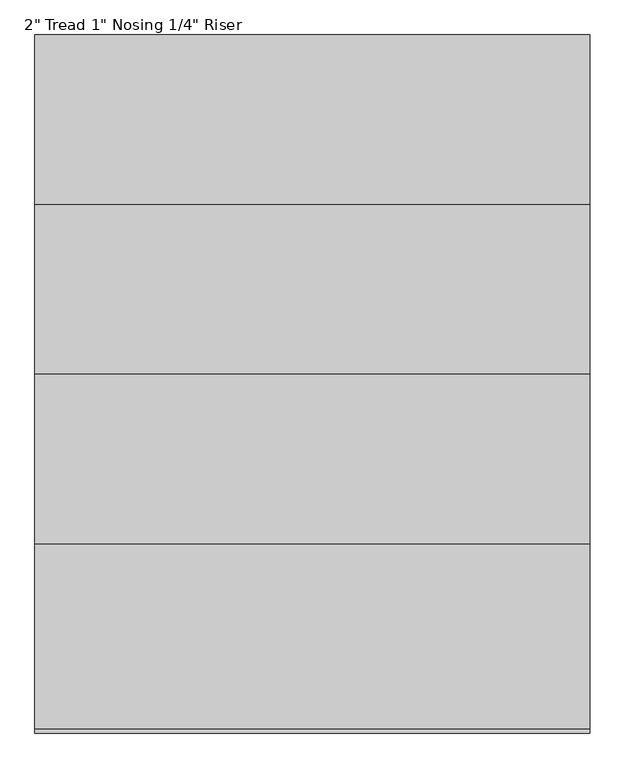
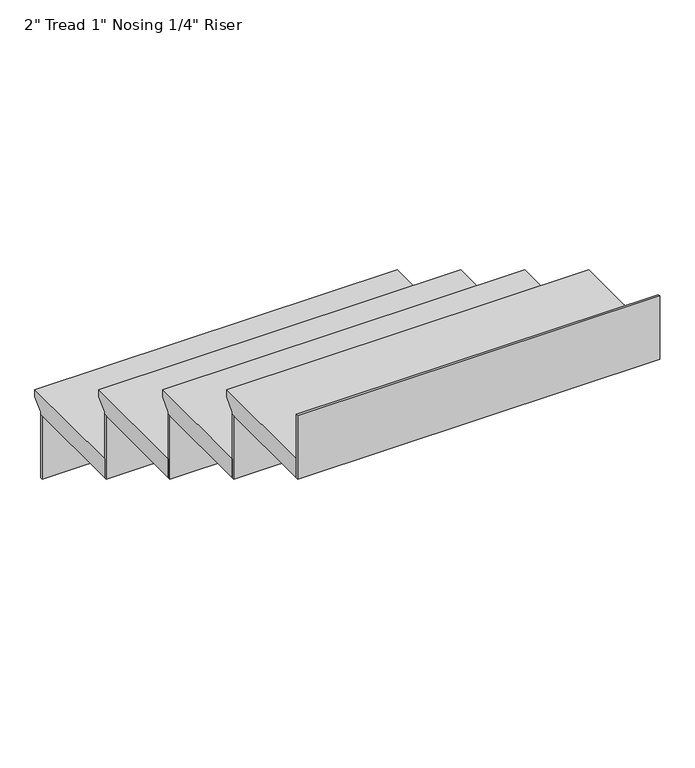
"""IFC4 building model written with IfcOpenShell, lengths in millimetres: stair flight geometry."""

from ifc_helpers import new_model, si_unit, frame, origin, place, context, project, spatial, polyline, outline, extrude, source, transform, mapped, element, save


def stair_flight_e8b6355c(model_context):
    return source(origin(), model_context, "Body", "SweptSolid", [
        extrude(outline(polyline([(22889.9216096, 36749.2839133), (23194.7216096, 36749.2839133), (23194.7216096, 36730.2339133), (23169.3216096, 36704.8339133), (23169.3216096, 36698.4839133), (22889.9216096, 36698.4839133), (22889.9216096, 36749.2839133)])), frame((-2398.2415084, 0.0, 0.0), z_axis=(1.0, 0.0, 0.0), x_axis=(0.0, 1.0, 0.0)), (0.0, 0.0, 1.0), 914.4),
        extrude(outline(polyline([(-2398.2415084, 23162.9716096), (-2398.2415084, 23169.3216096), (-1483.8415084, 23169.3216096), (-1483.8415084, 23162.9716096), (-2398.2415084, 23162.9716096)])), frame((0.0, 0.0, 36529.1505799), z_axis=(0.0, 0.0, 1.0), x_axis=(1.0, 0.0, 0.0)), (0.0, 0.0, 1.0), 169.3333333),
        extrude(outline(polyline([(-2398.2415084, 22883.5716096), (-2398.2415084, 22889.9216096), (-1483.8415084, 22889.9216096), (-1483.8415084, 22883.5716096), (-2398.2415084, 22883.5716096)])), frame((0.0, 0.0, 36698.4839133), z_axis=(0.0, 0.0, 1.0), x_axis=(1.0, 0.0, 0.0)), (0.0, 0.0, 1.0), 169.3333333),
        extrude(outline(polyline([(22610.5216096, 36918.6172466), (22915.3216096, 36918.6172466), (22915.3216096, 36899.5672466), (22889.9216096, 36874.1672466), (22889.9216096, 36867.8172466), (22610.5216096, 36867.8172466), (22610.5216096, 36918.6172466)])), frame((-2398.2415084, 0.0, 0.0), z_axis=(1.0, 0.0, 0.0), x_axis=(0.0, 1.0, 0.0)), (0.0, 0.0, 1.0), 914.4),
        extrude(outline(polyline([(-2398.2415084, 22604.1716096), (-2398.2415084, 22610.5216096), (-1483.8415084, 22610.5216096), (-1483.8415084, 22604.1716096), (-2398.2415084, 22604.1716096)])), frame((0.0, 0.0, 36867.8172466), z_axis=(0.0, 0.0, 1.0), x_axis=(1.0, 0.0, 0.0)), (0.0, 0.0, 1.0), 169.3333333),
        extrude(outline(polyline([(22331.1216096, 37087.9505799), (22635.9216096, 37087.9505799), (22635.9216096, 37068.9005799), (22610.5216096, 37043.5005799), (22610.5216096, 37037.1505799), (22331.1216096, 37037.1505799), (22331.1216096, 37087.9505799)])), frame((-2398.2415084, 0.0, 0.0), z_axis=(1.0, 0.0, 0.0), x_axis=(0.0, 1.0, 0.0)), (0.0, 0.0, 1.0), 914.4),
        extrude(outline(polyline([(-2398.2415084, 22324.7716096), (-2398.2415084, 22331.1216096), (-1483.8415084, 22331.1216096), (-1483.8415084, 22324.7716096), (-2398.2415084, 22324.7716096)])), frame((0.0, 0.0, 37037.1505799), z_axis=(0.0, 0.0, 1.0), x_axis=(1.0, 0.0, 0.0)), (0.0, 0.0, 1.0), 169.3333333),
        extrude(outline(polyline([(-2398.2415084, 22045.3716096), (-2398.2415084, 22051.7216096), (-1483.8415084, 22051.7216096), (-1483.8415084, 22045.3716096), (-2398.2415084, 22045.3716096)])), frame((0.0, 0.0, 37206.4839133), z_axis=(0.0, 0.0, 1.0), x_axis=(1.0, 0.0, 0.0)), (0.0, 0.0, 1.0), 169.3333333),
        extrude(outline(polyline([(22051.7216096, 37257.2839133), (22356.5216096, 37257.2839133), (22356.5216096, 37238.2339133), (22331.1216096, 37212.8339133), (22331.1216096, 37206.4839133), (22051.7216096, 37206.4839133), (22051.7216096, 37257.2839133)])), frame((-2398.2415084, 0.0, 0.0), z_axis=(1.0, 0.0, 0.0), x_axis=(0.0, 1.0, 0.0)), (0.0, 0.0, 1.0), 914.4),
    ])


if __name__ == "__main__":
    model = new_model("IFC4")
    model_context = context("Model", 3, world=origin())
    ifc_project = project(units=[si_unit("LENGTHUNIT", "METRE", prefix="MILLI")], contexts=[model_context])
    site = spatial("IfcSite", under=ifc_project)
    building = spatial("IfcBuilding", under=site)
    placement = place(None, origin())
    stair_flight_shape = stair_flight_e8b6355c(model_context)
    element("IfcStairFlight", 1, ObjectType="2\" Tread 1\" Nosing 1/4\" Riser", at=placement, inside=building, context=model_context, shape_type="MappedRepresentation", body=[
        mapped(stair_flight_shape, transform((0.0, 0.0, 0.0), x_axis=(1.0, 0.0, 0.0), y_axis=(0.0, 1.0, 0.0), z_axis=(0.0, 0.0, 1.0))),
    ])
    save(model, "model.ifc")
